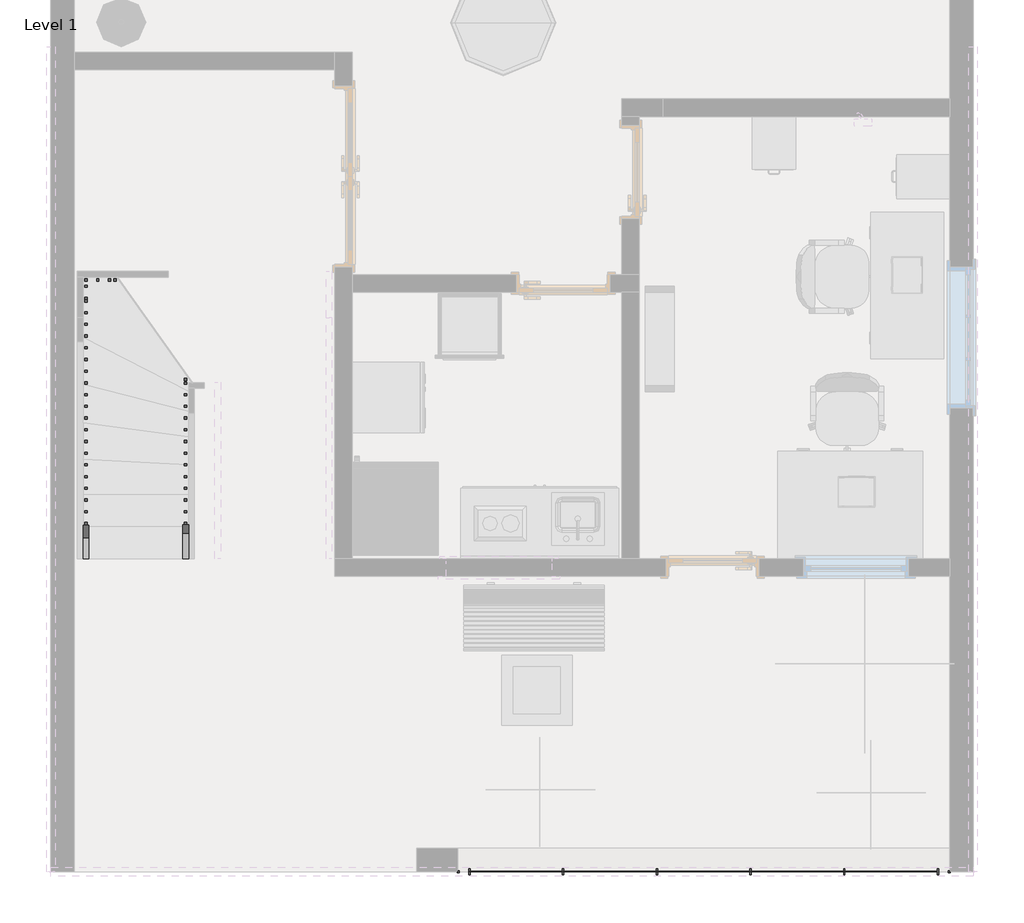
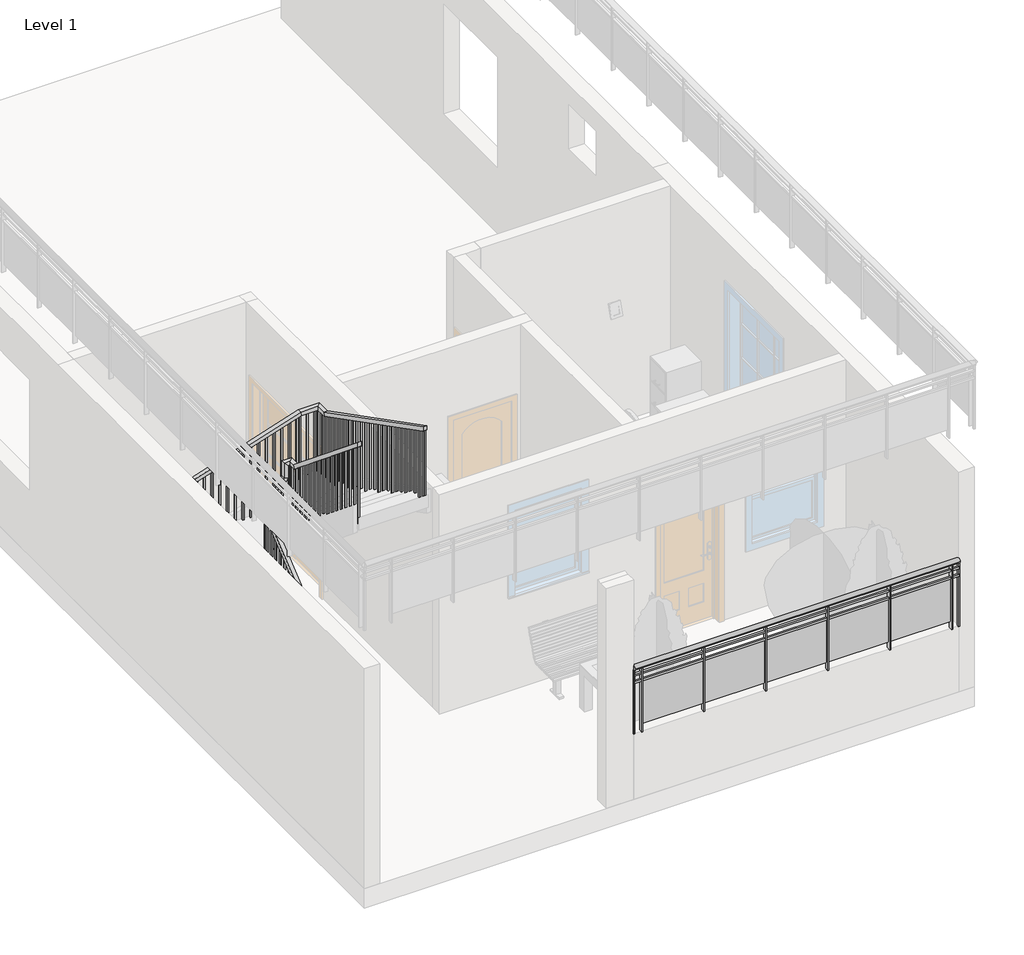
# One storey, part 2 of 4: 3 railings.
"""IFC4 building model written with IfcOpenShell, lengths in millimetres."""

from ifc_helpers import new_model, si_unit, point, frame, origin, place, context, project, spatial, polyline, ellipse_curve, trimmed, outline, extrude, faceted_brep, element, save
from ifc_brep_helpers import plane_surface, extruded_surface, advanced_brep

model = new_model("IFC4")

# Units and contexts
model_context = context("Model", 3, world=origin())
ifc_project = project(units=[si_unit("LENGTHUNIT", "METRE", prefix="MILLI")], contexts=[model_context])

# Site, building, storey
site = spatial("IfcSite", under=ifc_project)
building = spatial("IfcBuilding", under=site)
storey = spatial("IfcBuildingStorey", under=building, Name="Level 1", Elevation=0.0)

# Railings
placement = place(None, origin())
element("IfcRailing", 1, ObjectType="Glass Panel - Bottom Fill", at=placement, inside=storey, context=model_context, shape_type="SolidModel", body=[
    advanced_brep(
    [(-10033.9568901, -1887.378876, 1828.8), (-10033.9568901, -1963.578876, 1828.8), (-5766.7568901, -1887.378876, 1828.8), (-5766.7568901, -1963.578876, 1828.8)],
    [
        (0, 1, ellipse_curve(frame((-10033.9568901, -1925.478876, 1828.8), z_axis=(-1.0, 0.0, 0.0), x_axis=(0.0, -1.0, 0.0)), 38.1, 28.575)),
        (1, 0, ellipse_curve(frame((-10033.9568901, -1925.478876, 1828.8), z_axis=(-1.0, 0.0, 0.0), x_axis=(0.0, -1.0, 0.0)), 38.1, 28.575)),
        (2, 3, ellipse_curve(frame((-5766.7568901, -1925.478876, 1828.8), z_axis=(1.0, 0.0, 0.0), x_axis=(0.0, -1.0, 0.0)), 38.1, 28.575)),
        (3, 2, ellipse_curve(frame((-5766.7568901, -1925.478876, 1828.8), z_axis=(1.0, 0.0, 0.0), x_axis=(0.0, -1.0, 0.0)), 38.1, 28.575)),
        (0, 2),
        (3, 1),
    ],
    [
        plane_surface(frame((-10033.9568901, -1925.478876, 1828.8), z_axis=(-1.0, 0.0, 0.0), x_axis=(0.0, 1.0, 0.0))),
        plane_surface(frame((-5766.7568901, -1925.478876, 1828.8), z_axis=(1.0, 0.0, 0.0), x_axis=(0.0, 1.0, 0.0))),
        extruded_surface(trimmed(ellipse_curve(frame((-5766.7568901, -1925.478876, 1828.8), z_axis=(-1.0, 0.0, 0.0), x_axis=(0.0, -1.0, 0.0)), 38.1, 28.575), [point((-5766.7568901, -1887.378876, 1828.8))], [point((-5766.7568901, -1963.578876, 1828.8))], True, "CARTESIAN"), (-4267.2, 0.0, 0.0), 4267.2),
        extruded_surface(trimmed(ellipse_curve(frame((-5766.7568901, -1925.478876, 1828.8), z_axis=(-1.0, 0.0, 0.0), x_axis=(0.0, -1.0, 0.0)), 38.1, 28.575), [point((-5766.7568901, -1963.578876, 1828.8))], [point((-5766.7568901, -1887.378876, 1828.8))], True, "CARTESIAN"), (-4267.2, 0.0, 0.0), 4267.2),
    ],
    [
        (0, [[1, 2]]),
        (1, [[3, 4]]),
        (2, [[-1, 5, -4, 6]]),
        (3, [[-2, -6, -3, -5]]),
    ],
),
    extrude(outline(polyline([(-10033.9568901, -1938.178876), (-10033.9568901, -1912.778876), (-5766.7568901, -1912.778876), (-5766.7568901, -1938.178876), (-10033.9568901, -1938.178876)])), frame((0.0, 0.0, 1714.5), z_axis=(0.0, 0.0, 1.0), x_axis=(1.0, 0.0, 0.0)), (0.0, 0.0, 1.0), 25.4),
    extrude(outline(polyline([(-10033.9568901, -1938.178876), (-10033.9568901, -1912.778876), (-5766.7568901, -1912.778876), (-5766.7568901, -1938.178876), (-10033.9568901, -1938.178876)])), frame((0.0, 0.0, 1612.9), z_axis=(0.0, 0.0, 1.0), x_axis=(1.0, 0.0, 0.0)), (0.0, 0.0, 1.0), 25.4),
    extrude(outline(polyline([(-5874.7068901, -1950.878876), (-5874.7068901, -1900.078876), (-5862.0068901, -1900.078876), (-5862.0068901, -1950.878876), (-5874.7068901, -1950.878876)])), frame((0.0, 0.0, 914.4), z_axis=(0.0, 0.0, 1.0), x_axis=(1.0, 0.0, 0.0)), (0.0, 0.0, 1.0), 885.6788223),
    extrude(outline(polyline([(-6681.1568901, -1918.943719), (-5868.3568901, -1918.943719), (-5868.3568901, -1925.293719), (-6681.1568901, -1925.293719), (-6681.1568901, -1918.943719)])), frame((0.0, 0.0, 1016.0), z_axis=(0.0, 0.0, 1.0), x_axis=(1.0, 0.0, 0.0)), (0.0, 0.0, 1.0), 596.9),
    extrude(outline(polyline([(-6687.5068901, -1950.878876), (-6687.5068901, -1900.078876), (-6674.8068901, -1900.078876), (-6674.8068901, -1950.878876), (-6687.5068901, -1950.878876)])), frame((0.0, 0.0, 914.4), z_axis=(0.0, 0.0, 1.0), x_axis=(1.0, 0.0, 0.0)), (0.0, 0.0, 1.0), 885.6788223),
    extrude(outline(polyline([(-7493.9568901, -1918.943719), (-6681.1568901, -1918.943719), (-6681.1568901, -1925.293719), (-7493.9568901, -1925.293719), (-7493.9568901, -1918.943719)])), frame((0.0, 0.0, 1016.0), z_axis=(0.0, 0.0, 1.0), x_axis=(1.0, 0.0, 0.0)), (0.0, 0.0, 1.0), 596.9),
    extrude(outline(polyline([(-7500.3068901, -1950.878876), (-7500.3068901, -1900.078876), (-7487.6068901, -1900.078876), (-7487.6068901, -1950.878876), (-7500.3068901, -1950.878876)])), frame((0.0, 0.0, 914.4), z_axis=(0.0, 0.0, 1.0), x_axis=(1.0, 0.0, 0.0)), (0.0, 0.0, 1.0), 885.6788223),
    extrude(outline(polyline([(-8306.7568901, -1918.943719), (-7493.9568901, -1918.943719), (-7493.9568901, -1925.293719), (-8306.7568901, -1925.293719), (-8306.7568901, -1918.943719)])), frame((0.0, 0.0, 1016.0), z_axis=(0.0, 0.0, 1.0), x_axis=(1.0, 0.0, 0.0)), (0.0, 0.0, 1.0), 596.9),
    extrude(outline(polyline([(-8313.1068901, -1950.878876), (-8313.1068901, -1900.078876), (-8300.4068901, -1900.078876), (-8300.4068901, -1950.878876), (-8313.1068901, -1950.878876)])), frame((0.0, 0.0, 914.4), z_axis=(0.0, 0.0, 1.0), x_axis=(1.0, 0.0, 0.0)), (0.0, 0.0, 1.0), 885.6788223),
    extrude(outline(polyline([(-9119.5568901, -1918.943719), (-8306.7568901, -1918.943719), (-8306.7568901, -1925.293719), (-9119.5568901, -1925.293719), (-9119.5568901, -1918.943719)])), frame((0.0, 0.0, 1016.0), z_axis=(0.0, 0.0, 1.0), x_axis=(1.0, 0.0, 0.0)), (0.0, 0.0, 1.0), 596.9),
    extrude(outline(polyline([(-9125.9068901, -1950.878876), (-9125.9068901, -1900.078876), (-9113.2068901, -1900.078876), (-9113.2068901, -1950.878876), (-9125.9068901, -1950.878876)])), frame((0.0, 0.0, 914.4), z_axis=(0.0, 0.0, 1.0), x_axis=(1.0, 0.0, 0.0)), (0.0, 0.0, 1.0), 885.6788223),
    extrude(outline(polyline([(-9932.3568901, -1918.943719), (-9119.5568901, -1918.943719), (-9119.5568901, -1925.293719), (-9932.3568901, -1925.293719), (-9932.3568901, -1918.943719)])), frame((0.0, 0.0, 1016.0), z_axis=(0.0, 0.0, 1.0), x_axis=(1.0, 0.0, 0.0)), (0.0, 0.0, 1.0), 596.9),
    extrude(outline(polyline([(-9938.7068901, -1950.878876), (-9938.7068901, -1900.078876), (-9926.0068901, -1900.078876), (-9926.0068901, -1950.878876), (-9938.7068901, -1950.878876)])), frame((0.0, 0.0, 914.4), z_axis=(0.0, 0.0, 1.0), x_axis=(1.0, 0.0, 0.0)), (0.0, 0.0, 1.0), 885.6788223),
    extrude(outline(polyline([(-5779.4568901, -1935.003876), (-5779.4568901, -1915.953876), (-5760.4068901, -1915.953876), (-5760.4068901, -1935.003876), (-5779.4568901, -1935.003876)])), frame((0.0, 0.0, 914.4), z_axis=(0.0, 0.0, 1.0), x_axis=(1.0, 0.0, 0.0)), (0.0, 0.0, 1.0), 885.6788223),
    extrude(outline(polyline([(-10040.3068901, -1935.003876), (-10040.3068901, -1915.953876), (-10021.2568901, -1915.953876), (-10021.2568901, -1935.003876), (-10040.3068901, -1935.003876)])), frame((0.0, 0.0, 914.4), z_axis=(0.0, 0.0, 1.0), x_axis=(1.0, 0.0, 0.0)), (0.0, 0.0, 1.0), 885.6788223),
])
element("IfcRailing", 2, ObjectType="Handrail - Rectangular", at=placement, inside=storey, context=model_context, shape_type="SolidModel", body=[
    faceted_brep([(-12421.5568901, 792.321124, 1025.2529681), (-12421.5568901, 792.321124, 959.7067088), (-12370.7568901, 792.321124, 959.7067088), (-12370.7568901, 792.321124, 1025.2529681), (-12421.5568901, 2243.8528159, 2208.7848338), (-12421.5568901, 2294.6528159, 2184.659247), (-12370.7568901, 2294.6528159, 2184.659247), (-12370.7568901, 2243.8528159, 2208.7848338), (-12421.5568901, 2243.8528159, 2414.6281882), (-12421.5568901, 2294.6528159, 2363.8281882), (-12370.7568901, 2294.6528159, 2363.8281882), (-12370.7568901, 2243.8528159, 2414.6281882), (-12421.5568901, 2370.8528159, 2414.6281882), (-12421.5568901, 2370.8528159, 2363.8281882), (-12370.7568901, 2320.0528159, 2363.8281882), (-12370.7568901, 2320.0528159, 2414.6281882), (-12294.5568901, 2370.8528159, 2414.6281882), (-12265.4355563, 2370.8528159, 2363.8281882), (-12265.4355563, 2320.0528159, 2363.8281882), (-12294.5568901, 2320.0528159, 2414.6281882), (-12167.5568901, 2370.8528159, 2631.5051451), (-12116.7568901, 2370.8528159, 2617.7256424), (-12116.7568901, 2320.0528159, 2617.7256424), (-12167.5568901, 2320.0528159, 2631.5051451), (-12167.5568901, 2370.8528159, 2837.3484995), (-12116.7568901, 2370.8528159, 2786.5484995), (-12116.7568901, 2320.0528159, 2786.5484995), (-12167.5568901, 2320.0528159, 2837.3484995), (-12040.5568901, 2370.8528159, 2837.3484995), (-12040.5568901, 2370.8528159, 2786.5484995), (-12091.3568901, 2320.0528159, 2786.5484995), (-12091.3568901, 2320.0528159, 2837.3484995), (-12040.5568901, 2243.8528159, 2837.3484995), (-12040.5568901, 2225.7674028, 2786.5484995), (-12091.3568901, 2225.7674028, 2786.5484995), (-12091.3568901, 2243.8528159, 2837.3484995), (-12040.5568901, 792.321124, 4020.8803652), (-12091.3568901, 792.321124, 4020.8803652), (-12091.3568901, 792.321124, 3955.3341059), (-12040.5568901, 792.321124, 3955.3341059)], [[[0, 1, 2, 3]], [[1, 0, 4, 5]], [[2, 1, 5, 6]], [[3, 2, 6, 7]], [[0, 3, 7, 4]], [[5, 4, 8, 9]], [[6, 5, 9, 10]], [[7, 6, 10, 11]], [[4, 7, 11, 8]], [[9, 8, 12, 13]], [[10, 9, 13, 14]], [[11, 10, 14, 15]], [[8, 11, 15, 12]], [[13, 12, 16, 17]], [[14, 13, 17, 18]], [[15, 14, 18, 19]], [[12, 15, 19, 16]], [[17, 16, 20, 21]], [[18, 17, 21, 22]], [[19, 18, 22, 23]], [[16, 19, 23, 20]], [[21, 20, 24, 25]], [[22, 21, 25, 26]], [[23, 22, 26, 27]], [[20, 23, 27, 24]], [[25, 24, 28, 29]], [[26, 25, 29, 30]], [[27, 26, 30, 31]], [[24, 27, 31, 28]], [[29, 28, 32, 33]], [[30, 29, 33, 34]], [[31, 30, 34, 35]], [[28, 31, 35, 32]], [[36, 37, 38, 39]], [[33, 32, 36, 39]], [[34, 33, 39, 38]], [[35, 34, 38, 37]], [[32, 35, 37, 36]]]),
    extrude(outline(polyline([(882.5604595, 3881.7558784), (901.6104595, 3866.2231262), (901.6104595, 2878.6666667), (882.5604595, 2878.6666667), (882.5604595, 3881.7558784)])), frame((-12075.4818901, 0.0, 0.0), z_axis=(1.0, 0.0, 0.0), x_axis=(0.0, 1.0, 0.0)), (0.0, 0.0, 1.0), 19.05),
    extrude(outline(polyline([(984.1604595, 3798.9145334), (1003.2104595, 3783.3817813), (1003.2104595, 2878.6666667), (984.1604595, 2878.6666667), (984.1604595, 3798.9145334)])), frame((-12075.4818901, 0.0, 0.0), z_axis=(1.0, 0.0, 0.0), x_axis=(0.0, 1.0, 0.0)), (0.0, 0.0, 1.0), 19.05),
    extrude(outline(polyline([(1085.7604595, 3716.0731885), (1104.8104595, 3700.5404364), (1104.8104595, 2709.3333333), (1085.7604595, 2709.3333333), (1085.7604595, 3716.0731885)])), frame((-12075.4818901, 0.0, 0.0), z_axis=(1.0, 0.0, 0.0), x_axis=(0.0, 1.0, 0.0)), (0.0, 0.0, 1.0), 19.05),
    extrude(outline(polyline([(1187.3604595, 3633.2318436), (1206.4104595, 3617.6990914), (1206.4104595, 2709.3333333), (1187.3604595, 2709.3333333), (1187.3604595, 3633.2318436)])), frame((-12075.4818901, 0.0, 0.0), z_axis=(1.0, 0.0, 0.0), x_axis=(0.0, 1.0, 0.0)), (0.0, 0.0, 1.0), 19.05),
    extrude(outline(polyline([(1288.9604595, 3550.3904987), (1308.0104595, 3534.8577465), (1308.0104595, 2709.3333333), (1288.9604595, 2709.3333333), (1288.9604595, 3550.3904987)])), frame((-12075.4818901, 0.0, 0.0), z_axis=(1.0, 0.0, 0.0), x_axis=(0.0, 1.0, 0.0)), (0.0, 0.0, 1.0), 19.05),
    extrude(outline(polyline([(1390.5604595, 3467.5491538), (1409.6104595, 3452.0164016), (1409.6104595, 2540.0), (1390.5604595, 2540.0), (1390.5604595, 3467.5491538)])), frame((-12075.4818901, 0.0, 0.0), z_axis=(1.0, 0.0, 0.0), x_axis=(0.0, 1.0, 0.0)), (0.0, 0.0, 1.0), 19.05),
    extrude(outline(polyline([(1492.1604595, 3384.7078088), (1511.2104595, 3369.1750567), (1511.2104595, 2540.0), (1492.1604595, 2540.0), (1492.1604595, 3384.7078088)])), frame((-12075.4818901, 0.0, 0.0), z_axis=(1.0, 0.0, 0.0), x_axis=(0.0, 1.0, 0.0)), (0.0, 0.0, 1.0), 19.05),
    extrude(outline(polyline([(1593.7604595, 3301.8664639), (1612.8104595, 3286.3337117), (1612.8104595, 2540.0), (1593.7604595, 2540.0), (1593.7604595, 3301.8664639)])), frame((-12075.4818901, 0.0, 0.0), z_axis=(1.0, 0.0, 0.0), x_axis=(0.0, 1.0, 0.0)), (0.0, 0.0, 1.0), 19.05),
    extrude(outline(polyline([(1695.3604595, 3219.025119), (1714.4104595, 3203.4923668), (1714.4104595, 2370.6666667), (1695.3604595, 2370.6666667), (1695.3604595, 3219.025119)])), frame((-12075.4818901, 0.0, 0.0), z_axis=(1.0, 0.0, 0.0), x_axis=(0.0, 1.0, 0.0)), (0.0, 0.0, 1.0), 19.05),
    extrude(outline(polyline([(1796.9604595, 3136.1837741), (1816.0104595, 3120.6510219), (1816.0104595, 2370.6666667), (1796.9604595, 2370.6666667), (1796.9604595, 3136.1837741)])), frame((-12075.4818901, 0.0, 0.0), z_axis=(1.0, 0.0, 0.0), x_axis=(0.0, 1.0, 0.0)), (0.0, 0.0, 1.0), 19.05),
    extrude(outline(polyline([(1898.5604595, 3053.3424291), (1917.6104595, 3037.809677), (1917.6104595, 2201.3333333), (1898.5604595, 2201.3333333), (1898.5604595, 3053.3424291)])), frame((-12075.4818901, 0.0, 0.0), z_axis=(1.0, 0.0, 0.0), x_axis=(0.0, 1.0, 0.0)), (0.0, 0.0, 1.0), 19.05),
    extrude(outline(polyline([(2000.1604595, 2970.5010842), (2019.2104595, 2954.9683321), (2019.2104595, 2201.3333333), (2000.1604595, 2201.3333333), (2000.1604595, 2970.5010842)])), frame((-12075.4818901, 0.0, 0.0), z_axis=(1.0, 0.0, 0.0), x_axis=(0.0, 1.0, 0.0)), (0.0, 0.0, 1.0), 19.05),
    extrude(outline(polyline([(2101.7604595, 2887.6597393), (2120.8104595, 2872.1269871), (2120.8104595, 2032.0), (2101.7604595, 2032.0), (2101.7604595, 2887.6597393)])), frame((-12075.4818901, 0.0, 0.0), z_axis=(1.0, 0.0, 0.0), x_axis=(0.0, 1.0, 0.0)), (0.0, 0.0, 1.0), 19.05),
    extrude(outline(polyline([(2203.3604595, 2804.8183944), (2222.4104595, 2789.2856422), (2222.4104595, 2032.0), (2203.3604595, 2032.0), (2203.3604595, 2804.8183944)])), frame((-12075.4818901, 0.0, 0.0), z_axis=(1.0, 0.0, 0.0), x_axis=(0.0, 1.0, 0.0)), (0.0, 0.0, 1.0), 19.05),
    extrude(outline(polyline([(2529.115018, -12168.6459863), (2496.5834745, -12187.6959863), (1524.0, -12187.6959863), (1524.0, -12168.6459863), (2529.115018, -12168.6459863)])), frame((0.0, 2335.9278159, 0.0), z_axis=(0.0, 1.0, 0.0), x_axis=(0.0, 0.0, 1.0)), (0.0, 0.0, 1.0), 19.05),
    extrude(outline(polyline([(2355.6134525, -12270.2459863), (2323.0819089, -12289.2959863), (1524.0, -12289.2959863), (1524.0, -12270.2459863), (2355.6134525, -12270.2459863)])), frame((0.0, 2335.9278159, 0.0), z_axis=(0.0, 1.0, 0.0), x_axis=(0.0, 0.0, 1.0)), (0.0, 0.0, 1.0), 19.05),
    extrude(outline(polyline([(2205.196124, 2111.7191617), (2224.246124, 2127.2519138), (2224.246124, 1016.0), (2205.196124, 1016.0), (2205.196124, 2111.7191617)])), frame((-12405.6818901, 0.0, 0.0), z_axis=(1.0, 0.0, 0.0), x_axis=(0.0, 1.0, 0.0)), (0.0, 0.0, 1.0), 19.05),
    extrude(outline(polyline([(2103.596124, 2028.8778167), (2122.646124, 2044.4105689), (2122.646124, 1016.0), (2103.596124, 1016.0), (2103.596124, 2028.8778167)])), frame((-12405.6818901, 0.0, 0.0), z_axis=(1.0, 0.0, 0.0), x_axis=(0.0, 1.0, 0.0)), (0.0, 0.0, 1.0), 19.05),
    extrude(outline(polyline([(2001.996124, 1946.0364718), (2021.046124, 1961.569224), (2021.046124, 846.6666667), (2001.996124, 846.6666667), (2001.996124, 1946.0364718)])), frame((-12405.6818901, 0.0, 0.0), z_axis=(1.0, 0.0, 0.0), x_axis=(0.0, 1.0, 0.0)), (0.0, 0.0, 1.0), 19.05),
    extrude(outline(polyline([(1900.396124, 1863.1951269), (1919.446124, 1878.7278791), (1919.446124, 846.6666667), (1900.396124, 846.6666667), (1900.396124, 1863.1951269)])), frame((-12405.6818901, 0.0, 0.0), z_axis=(1.0, 0.0, 0.0), x_axis=(0.0, 1.0, 0.0)), (0.0, 0.0, 1.0), 19.05),
    extrude(outline(polyline([(1798.796124, 1780.353782), (1817.846124, 1795.8865341), (1817.846124, 677.3333333), (1798.796124, 677.3333333), (1798.796124, 1780.353782)])), frame((-12405.6818901, 0.0, 0.0), z_axis=(1.0, 0.0, 0.0), x_axis=(0.0, 1.0, 0.0)), (0.0, 0.0, 1.0), 19.05),
    extrude(outline(polyline([(1697.196124, 1697.5124371), (1716.246124, 1713.0451892), (1716.246124, 677.3333333), (1697.196124, 677.3333333), (1697.196124, 1697.5124371)])), frame((-12405.6818901, 0.0, 0.0), z_axis=(1.0, 0.0, 0.0), x_axis=(0.0, 1.0, 0.0)), (0.0, 0.0, 1.0), 19.05),
    extrude(outline(polyline([(1595.596124, 1614.6710921), (1614.646124, 1630.2038443), (1614.646124, 508.0), (1595.596124, 508.0), (1595.596124, 1614.6710921)])), frame((-12405.6818901, 0.0, 0.0), z_axis=(1.0, 0.0, 0.0), x_axis=(0.0, 1.0, 0.0)), (0.0, 0.0, 1.0), 19.05),
    extrude(outline(polyline([(1493.996124, 1531.8297472), (1513.046124, 1547.3624994), (1513.046124, 508.0), (1493.996124, 508.0), (1493.996124, 1531.8297472)])), frame((-12405.6818901, 0.0, 0.0), z_axis=(1.0, 0.0, 0.0), x_axis=(0.0, 1.0, 0.0)), (0.0, 0.0, 1.0), 19.05),
    extrude(outline(polyline([(1392.396124, 1448.9884023), (1411.446124, 1464.5211545), (1411.446124, 508.0), (1392.396124, 508.0), (1392.396124, 1448.9884023)])), frame((-12405.6818901, 0.0, 0.0), z_axis=(1.0, 0.0, 0.0), x_axis=(0.0, 1.0, 0.0)), (0.0, 0.0, 1.0), 19.05),
    extrude(outline(polyline([(1290.796124, 1366.1470574), (1309.846124, 1381.6798095), (1309.846124, 338.6666667), (1290.796124, 338.6666667), (1290.796124, 1366.1470574)])), frame((-12405.6818901, 0.0, 0.0), z_axis=(1.0, 0.0, 0.0), x_axis=(0.0, 1.0, 0.0)), (0.0, 0.0, 1.0), 19.05),
    extrude(outline(polyline([(1189.196124, 1283.3057124), (1208.246124, 1298.8384646), (1208.246124, 338.6666667), (1189.196124, 338.6666667), (1189.196124, 1283.3057124)])), frame((-12405.6818901, 0.0, 0.0), z_axis=(1.0, 0.0, 0.0), x_axis=(0.0, 1.0, 0.0)), (0.0, 0.0, 1.0), 19.05),
    extrude(outline(polyline([(1087.596124, 1200.4643675), (1106.646124, 1215.9971197), (1106.646124, 338.6666667), (1087.596124, 338.6666667), (1087.596124, 1200.4643675)])), frame((-12405.6818901, 0.0, 0.0), z_axis=(1.0, 0.0, 0.0), x_axis=(0.0, 1.0, 0.0)), (0.0, 0.0, 1.0), 19.05),
    extrude(outline(polyline([(985.996124, 1117.6230226), (1005.046124, 1133.1557748), (1005.046124, 169.3333333), (985.996124, 169.3333333), (985.996124, 1117.6230226)])), frame((-12405.6818901, 0.0, 0.0), z_axis=(1.0, 0.0, 0.0), x_axis=(0.0, 1.0, 0.0)), (0.0, 0.0, 1.0), 19.05),
    extrude(outline(polyline([(884.396124, 1034.7816777), (903.446124, 1050.3144298), (903.446124, 169.3333333), (884.396124, 169.3333333), (884.396124, 1034.7816777)])), frame((-12405.6818901, 0.0, 0.0), z_axis=(1.0, 0.0, 0.0), x_axis=(0.0, 1.0, 0.0)), (0.0, 0.0, 1.0), 19.05),
    extrude(outline(polyline([(-12075.4818901, 2324.0104595), (-12056.4318901, 2324.0104595), (-12056.4318901, 2304.9604595), (-12075.4818901, 2304.9604595), (-12075.4818901, 2324.0104595)])), frame((0.0, 0.0, 1862.6666667), z_axis=(0.0, 0.0, 1.0), x_axis=(1.0, 0.0, 0.0)), (0.0, 0.0, 1.0), 923.8818329),
    extrude(outline(polyline([(-12075.4818901, 2335.9278159), (-12075.4818901, 2354.9778159), (-12056.4318901, 2354.9778159), (-12056.4318901, 2335.9278159), (-12075.4818901, 2335.9278159)])), frame((0.0, 0.0, 1862.6666667), z_axis=(0.0, 0.0, 1.0), x_axis=(1.0, 0.0, 0.0)), (0.0, 0.0, 1.0), 923.8818329),
    extrude(outline(polyline([(-12090.2677938, 2335.9278159), (-12090.2677938, 2354.9778159), (-12071.2177938, 2354.9778159), (-12071.2177938, 2335.9278159), (-12090.2677938, 2335.9278159)])), frame((0.0, 0.0, 1693.3333333), z_axis=(0.0, 0.0, 1.0), x_axis=(1.0, 0.0, 0.0)), (0.0, 0.0, 1.0), 1093.2151662),
    extrude(outline(polyline([(-12390.8959863, 2335.9278159), (-12390.8959863, 2354.9778159), (-12371.8459863, 2354.9778159), (-12371.8459863, 2335.9278159), (-12390.8959863, 2335.9278159)])), frame((0.0, 0.0, 1354.6666667), z_axis=(0.0, 0.0, 1.0), x_axis=(1.0, 0.0, 0.0)), (0.0, 0.0, 1.0), 1009.1615215),
    extrude(outline(polyline([(-12386.6318901, 2335.9278159), (-12405.6818901, 2335.9278159), (-12405.6818901, 2354.9778159), (-12386.6318901, 2354.9778159), (-12386.6318901, 2335.9278159)])), frame((0.0, 0.0, 1185.3333333), z_axis=(0.0, 0.0, 1.0), x_axis=(1.0, 0.0, 0.0)), (0.0, 0.0, 1.0), 1178.4948549),
    extrude(outline(polyline([(-12386.6318901, 2304.9604595), (-12405.6818901, 2304.9604595), (-12405.6818901, 2324.0104595), (-12386.6318901, 2324.0104595), (-12386.6318901, 2304.9604595)])), frame((0.0, 0.0, 1185.3333333), z_axis=(0.0, 0.0, 1.0), x_axis=(1.0, 0.0, 0.0)), (0.0, 0.0, 1.0), 1178.4948549),
    extrude(outline(polyline([(792.321124, 3955.3341059), (811.371124, 3939.8013537), (811.371124, 2878.6666667), (792.321124, 2878.6666667), (792.321124, 3955.3341059)])), frame((-12075.4818901, 0.0, 0.0), z_axis=(1.0, 0.0, 0.0), x_axis=(0.0, 1.0, 0.0)), (0.0, 0.0, 1.0), 19.05),
    extrude(outline(polyline([(792.321124, 959.7067088), (811.371124, 975.239461), (811.371124, 169.3333333), (792.321124, 169.3333333), (792.321124, 959.7067088)])), frame((-12405.6818901, 0.0, 0.0), z_axis=(1.0, 0.0, 0.0), x_axis=(0.0, 1.0, 0.0)), (0.0, 0.0, 1.0), 19.05),
])
element("IfcRailing", 3, ObjectType="Handrail - Rectangular", at=placement, inside=storey, context=model_context, shape_type="SolidModel", body=[
    faceted_brep([(-13285.1568901, 792.321124, 1109.0771751), (-13285.1568901, 792.321124, 1051.9280057), (-13234.3568901, 792.321124, 1051.9280057), (-13234.3568901, 792.321124, 1109.0771751), (-13285.1568901, 3052.3029805, 2273.7644996), (-13285.1568901, 3064.6230318, 2222.9644996), (-13234.3568901, 3064.6230318, 2222.9644996), (-13234.3568901, 3052.3029805, 2273.7644996), (-13285.1568901, 3234.4528159, 2273.7644996), (-13285.1568901, 3234.4528159, 2222.9644996), (-13234.3568901, 3183.6528159, 2222.9644996), (-13234.3568901, 3183.6528159, 2273.7644996), (-13008.0029375, 3234.4528159, 2273.7644996), (-13000.0523613, 3234.4528159, 2222.9644996), (-13000.0523613, 3183.6528159, 2222.9644996), (-13008.0029375, 3183.6528159, 2273.7644996), (-11454.1108427, 3234.4528159, 2772.3688337), (-11446.1602666, 3234.4528159, 2721.5688337), (-11446.1602666, 3183.6528159, 2721.5688337), (-11454.1108427, 3183.6528159, 2772.3688337), (-11176.9568901, 3234.4528159, 2772.3688337), (-11176.9568901, 3234.4528159, 2721.5688337), (-11227.7568901, 3183.6528159, 2721.5688337), (-11227.7568901, 3183.6528159, 2772.3688337), (-11176.9568901, 3052.3029805, 2772.3688337), (-11176.9568901, 3039.9829292, 2721.5688337), (-11227.7568901, 3039.9829292, 2721.5688337), (-11227.7568901, 3052.3029805, 2772.3688337), (-11176.9568901, 792.321124, 3937.0561582), (-11227.7568901, 792.321124, 3937.0561582), (-11227.7568901, 792.321124, 3879.9069889), (-11176.9568901, 792.321124, 3879.9069889)], [[[0, 1, 2, 3]], [[1, 0, 4, 5]], [[2, 1, 5, 6]], [[3, 2, 6, 7]], [[0, 3, 7, 4]], [[5, 4, 8, 9]], [[6, 5, 9, 10]], [[7, 6, 10, 11]], [[4, 7, 11, 8]], [[9, 8, 12, 13]], [[10, 9, 13, 14]], [[11, 10, 14, 15]], [[8, 11, 15, 12]], [[13, 12, 16, 17]], [[14, 13, 17, 18]], [[15, 14, 18, 19]], [[12, 15, 19, 16]], [[17, 16, 20, 21]], [[18, 17, 21, 22]], [[19, 18, 22, 23]], [[16, 19, 23, 20]], [[21, 20, 24, 25]], [[22, 21, 25, 26]], [[23, 22, 26, 27]], [[20, 23, 27, 24]], [[28, 29, 30, 31]], [[25, 24, 28, 31]], [[26, 25, 31, 30]], [[27, 26, 30, 29]], [[24, 27, 29, 28]]]),
    extrude(outline(polyline([(826.6279805, 3862.2268642), (826.6279805, 2878.6666667), (807.5779805, 2878.6666667), (807.5779805, 3872.0443296), (826.6279805, 3862.2268642)])), frame((-11211.8818901, 0.0, 0.0), z_axis=(1.0, 0.0, 0.0), x_axis=(0.0, 1.0, 0.0)), (0.0, 0.0, 1.0), 19.05),
    extrude(outline(polyline([(928.2279805, 3809.8670491), (928.2279805, 2878.6666667), (909.1779805, 2878.6666667), (909.1779805, 3819.6845145), (928.2279805, 3809.8670491)])), frame((-11211.8818901, 0.0, 0.0), z_axis=(1.0, 0.0, 0.0), x_axis=(0.0, 1.0, 0.0)), (0.0, 0.0, 1.0), 19.05),
    extrude(outline(polyline([(1029.8279805, 3757.507234), (1029.8279805, 2878.6666667), (1010.7779805, 2878.6666667), (1010.7779805, 3767.3246993), (1029.8279805, 3757.507234)])), frame((-11211.8818901, 0.0, 0.0), z_axis=(1.0, 0.0, 0.0), x_axis=(0.0, 1.0, 0.0)), (0.0, 0.0, 1.0), 19.05),
    extrude(outline(polyline([(1131.4279805, 3705.1474189), (1131.4279805, 2709.3333333), (1112.3779805, 2709.3333333), (1112.3779805, 3714.9648842), (1131.4279805, 3705.1474189)])), frame((-11211.8818901, 0.0, 0.0), z_axis=(1.0, 0.0, 0.0), x_axis=(0.0, 1.0, 0.0)), (0.0, 0.0, 1.0), 19.05),
    extrude(outline(polyline([(1233.0279805, 3652.7876038), (1233.0279805, 2709.3333333), (1213.9779805, 2709.3333333), (1213.9779805, 3662.6050691), (1233.0279805, 3652.7876038)])), frame((-11211.8818901, 0.0, 0.0), z_axis=(1.0, 0.0, 0.0), x_axis=(0.0, 1.0, 0.0)), (0.0, 0.0, 1.0), 19.05),
    extrude(outline(polyline([(1334.6279805, 3600.4277887), (1334.6279805, 2709.3333333), (1315.5779805, 2709.3333333), (1315.5779805, 3610.245254), (1334.6279805, 3600.4277887)])), frame((-11211.8818901, 0.0, 0.0), z_axis=(1.0, 0.0, 0.0), x_axis=(0.0, 1.0, 0.0)), (0.0, 0.0, 1.0), 19.05),
    extrude(outline(polyline([(1436.2279805, 3548.0679735), (1436.2279805, 2540.0), (1417.1779805, 2540.0), (1417.1779805, 3557.8854389), (1436.2279805, 3548.0679735)])), frame((-11211.8818901, 0.0, 0.0), z_axis=(1.0, 0.0, 0.0), x_axis=(0.0, 1.0, 0.0)), (0.0, 0.0, 1.0), 19.05),
    extrude(outline(polyline([(1537.8279805, 3495.7081584), (1537.8279805, 2540.0), (1518.7779805, 2540.0), (1518.7779805, 3505.5256238), (1537.8279805, 3495.7081584)])), frame((-11211.8818901, 0.0, 0.0), z_axis=(1.0, 0.0, 0.0), x_axis=(0.0, 1.0, 0.0)), (0.0, 0.0, 1.0), 19.05),
    extrude(outline(polyline([(1639.4279805, 3443.3483433), (1639.4279805, 2540.0), (1620.3779805, 2540.0), (1620.3779805, 3453.1658086), (1639.4279805, 3443.3483433)])), frame((-11211.8818901, 0.0, 0.0), z_axis=(1.0, 0.0, 0.0), x_axis=(0.0, 1.0, 0.0)), (0.0, 0.0, 1.0), 19.05),
    extrude(outline(polyline([(1741.0279805, 3390.9885282), (1741.0279805, 2370.6666667), (1721.9779805, 2370.6666667), (1721.9779805, 3400.8059935), (1741.0279805, 3390.9885282)])), frame((-11211.8818901, 0.0, 0.0), z_axis=(1.0, 0.0, 0.0), x_axis=(0.0, 1.0, 0.0)), (0.0, 0.0, 1.0), 19.05),
    extrude(outline(polyline([(1842.6279805, 3338.6287131), (1842.6279805, 2370.6666667), (1823.5779805, 2370.6666667), (1823.5779805, 3348.4461784), (1842.6279805, 3338.6287131)])), frame((-11211.8818901, 0.0, 0.0), z_axis=(1.0, 0.0, 0.0), x_axis=(0.0, 1.0, 0.0)), (0.0, 0.0, 1.0), 19.05),
    extrude(outline(polyline([(1944.2279805, 3286.268898), (1944.2279805, 2370.6666667), (1925.1779805, 2370.6666667), (1925.1779805, 3296.0863633), (1944.2279805, 3286.268898)])), frame((-11211.8818901, 0.0, 0.0), z_axis=(1.0, 0.0, 0.0), x_axis=(0.0, 1.0, 0.0)), (0.0, 0.0, 1.0), 19.05),
    extrude(outline(polyline([(2045.8279805, 3233.9090828), (2045.8279805, 2201.3333333), (2026.7779805, 2201.3333333), (2026.7779805, 3243.7265482), (2045.8279805, 3233.9090828)])), frame((-11211.8818901, 0.0, 0.0), z_axis=(1.0, 0.0, 0.0), x_axis=(0.0, 1.0, 0.0)), (0.0, 0.0, 1.0), 19.05),
    extrude(outline(polyline([(2147.4279805, 3181.5492677), (2147.4279805, 2201.3333333), (2128.3779805, 2201.3333333), (2128.3779805, 3191.3667331), (2147.4279805, 3181.5492677)])), frame((-11211.8818901, 0.0, 0.0), z_axis=(1.0, 0.0, 0.0), x_axis=(0.0, 1.0, 0.0)), (0.0, 0.0, 1.0), 19.05),
    extrude(outline(polyline([(2249.0279805, 3129.1894526), (2249.0279805, 2201.3333333), (2229.9779805, 2201.3333333), (2229.9779805, 3139.0069179), (2249.0279805, 3129.1894526)])), frame((-11211.8818901, 0.0, 0.0), z_axis=(1.0, 0.0, 0.0), x_axis=(0.0, 1.0, 0.0)), (0.0, 0.0, 1.0), 19.05),
    extrude(outline(polyline([(2350.6279805, 3076.8296375), (2350.6279805, 2032.0), (2331.5779805, 2032.0), (2331.5779805, 3086.6471028), (2350.6279805, 3076.8296375)])), frame((-11211.8818901, 0.0, 0.0), z_axis=(1.0, 0.0, 0.0), x_axis=(0.0, 1.0, 0.0)), (0.0, 0.0, 1.0), 19.05),
    extrude(outline(polyline([(2452.2279805, 3024.4698224), (2452.2279805, 2032.0), (2433.1779805, 2032.0), (2433.1779805, 3034.2872877), (2452.2279805, 3024.4698224)])), frame((-11211.8818901, 0.0, 0.0), z_axis=(1.0, 0.0, 0.0), x_axis=(0.0, 1.0, 0.0)), (0.0, 0.0, 1.0), 19.05),
    extrude(outline(polyline([(2553.8279805, 2972.1100073), (2553.8279805, 2032.0), (2534.7779805, 2032.0), (2534.7779805, 2981.9274726), (2553.8279805, 2972.1100073)])), frame((-11211.8818901, 0.0, 0.0), z_axis=(1.0, 0.0, 0.0), x_axis=(0.0, 1.0, 0.0)), (0.0, 0.0, 1.0), 19.05),
    extrude(outline(polyline([(2655.4279805, 2919.7501921), (2655.4279805, 2032.0), (2636.3779805, 2032.0), (2636.3779805, 2929.5676575), (2655.4279805, 2919.7501921)])), frame((-11211.8818901, 0.0, 0.0), z_axis=(1.0, 0.0, 0.0), x_axis=(0.0, 1.0, 0.0)), (0.0, 0.0, 1.0), 19.05),
    extrude(outline(polyline([(2757.0279805, 2867.390377), (2757.0279805, 1862.6666667), (2737.9779805, 1862.6666667), (2737.9779805, 2877.2078424), (2757.0279805, 2867.390377)])), frame((-11211.8818901, 0.0, 0.0), z_axis=(1.0, 0.0, 0.0), x_axis=(0.0, 1.0, 0.0)), (0.0, 0.0, 1.0), 19.05),
    extrude(outline(polyline([(2858.6279805, 2815.0305619), (2858.6279805, 1862.6666667), (2839.5779805, 1862.6666667), (2839.5779805, 2824.8480272), (2858.6279805, 2815.0305619)])), frame((-11211.8818901, 0.0, 0.0), z_axis=(1.0, 0.0, 0.0), x_axis=(0.0, 1.0, 0.0)), (0.0, 0.0, 1.0), 19.05),
    extrude(outline(polyline([(2960.2279805, 2762.6707468), (2960.2279805, 1862.6666667), (2941.1779805, 1862.6666667), (2941.1779805, 2772.4882121), (2960.2279805, 2762.6707468)])), frame((-11211.8818901, 0.0, 0.0), z_axis=(1.0, 0.0, 0.0), x_axis=(0.0, 1.0, 0.0)), (0.0, 0.0, 1.0), 19.05),
    extrude(outline(polyline([(-11192.8318901, 3116.9778159), (-11192.8318901, 3097.9278159), (-11211.8818901, 3097.9278159), (-11211.8818901, 3116.9778159), (-11192.8318901, 3116.9778159)])), frame((0.0, 0.0, 1862.6666667), z_axis=(0.0, 0.0, 1.0), x_axis=(1.0, 0.0, 0.0)), (0.0, 0.0, 1.0), 858.902167),
    extrude(outline(polyline([(-11260.4358427, 3218.5778159), (-11241.3858427, 3218.5778159), (-11241.3858427, 3199.5278159), (-11260.4358427, 3199.5278159), (-11260.4358427, 3218.5778159)])), frame((0.0, 0.0, 1862.6666667), z_axis=(0.0, 0.0, 1.0), x_axis=(1.0, 0.0, 0.0)), (0.0, 0.0, 1.0), 858.902167),
    extrude(outline(polyline([(-11362.0358427, 3218.5778159), (-11342.9858427, 3218.5778159), (-11342.9858427, 3199.5278159), (-11362.0358427, 3199.5278159), (-11362.0358427, 3218.5778159)])), frame((0.0, 0.0, 1862.6666667), z_axis=(0.0, 0.0, 1.0), x_axis=(1.0, 0.0, 0.0)), (0.0, 0.0, 1.0), 858.902167),
    extrude(outline(polyline([(2706.3697564, -11493.5279375), (1693.3333333, -11493.5279375), (1693.3333333, -11474.4779375), (2712.4824155, -11474.4779375), (2706.3697564, -11493.5279375)])), frame((0.0, 3199.5278159, 0.0), z_axis=(0.0, 1.0, 0.0), x_axis=(0.0, 0.0, 1.0)), (0.0, 0.0, 1.0), 19.05),
    extrude(outline(polyline([(2673.7689082, -11595.1279375), (1693.3333333, -11595.1279375), (1693.3333333, -11576.0779375), (2679.8815673, -11576.0779375), (2673.7689082, -11595.1279375)])), frame((0.0, 3199.5278159, 0.0), z_axis=(0.0, 1.0, 0.0), x_axis=(0.0, 0.0, 1.0)), (0.0, 0.0, 1.0), 19.05),
    extrude(outline(polyline([(2641.16806, -11696.7279375), (1693.3333333, -11696.7279375), (1693.3333333, -11677.6779375), (2647.280719, -11677.6779375), (2641.16806, -11696.7279375)])), frame((0.0, 3199.5278159, 0.0), z_axis=(0.0, 1.0, 0.0), x_axis=(0.0, 0.0, 1.0)), (0.0, 0.0, 1.0), 19.05),
    extrude(outline(polyline([(2608.5672118, -11798.3279375), (1693.3333333, -11798.3279375), (1693.3333333, -11779.2779375), (2614.6798708, -11779.2779375), (2608.5672118, -11798.3279375)])), frame((0.0, 3199.5278159, 0.0), z_axis=(0.0, 1.0, 0.0), x_axis=(0.0, 0.0, 1.0)), (0.0, 0.0, 1.0), 19.05),
    extrude(outline(polyline([(2575.9663635, -11899.9279375), (1693.3333333, -11899.9279375), (1693.3333333, -11880.8779375), (2582.0790226, -11880.8779375), (2575.9663635, -11899.9279375)])), frame((0.0, 3199.5278159, 0.0), z_axis=(0.0, 1.0, 0.0), x_axis=(0.0, 0.0, 1.0)), (0.0, 0.0, 1.0), 19.05),
    extrude(outline(polyline([(2543.3655153, -12001.5279375), (1693.3333333, -12001.5279375), (1693.3333333, -11982.4779375), (2549.4781744, -11982.4779375), (2543.3655153, -12001.5279375)])), frame((0.0, 3199.5278159, 0.0), z_axis=(0.0, 1.0, 0.0), x_axis=(0.0, 0.0, 1.0)), (0.0, 0.0, 1.0), 19.05),
    extrude(outline(polyline([(2510.7646671, -12103.1279375), (1524.0, -12103.1279375), (1524.0, -12084.0779375), (2516.8773261, -12084.0779375), (2510.7646671, -12103.1279375)])), frame((0.0, 3199.5278159, 0.0), z_axis=(0.0, 1.0, 0.0), x_axis=(0.0, 0.0, 1.0)), (0.0, 0.0, 1.0), 19.05),
    extrude(outline(polyline([(2478.1638189, -12204.7279375), (1524.0, -12204.7279375), (1524.0, -12185.6779375), (2484.2764779, -12185.6779375), (2478.1638189, -12204.7279375)])), frame((0.0, 3199.5278159, 0.0), z_axis=(0.0, 1.0, 0.0), x_axis=(0.0, 0.0, 1.0)), (0.0, 0.0, 1.0), 19.05),
    extrude(outline(polyline([(2445.5629706, -12306.3279375), (1524.0, -12306.3279375), (1524.0, -12287.2779375), (2451.6756297, -12287.2779375), (2445.5629706, -12306.3279375)])), frame((0.0, 3199.5278159, 0.0), z_axis=(0.0, 1.0, 0.0), x_axis=(0.0, 0.0, 1.0)), (0.0, 0.0, 1.0), 19.05),
    extrude(outline(polyline([(2412.9621224, -12407.9279375), (1524.0, -12407.9279375), (1524.0, -12388.8779375), (2419.0747814, -12388.8779375), (2412.9621224, -12407.9279375)])), frame((0.0, 3199.5278159, 0.0), z_axis=(0.0, 1.0, 0.0), x_axis=(0.0, 0.0, 1.0)), (0.0, 0.0, 1.0), 19.05),
    extrude(outline(polyline([(2380.3612742, -12509.5279375), (1354.6666667, -12509.5279375), (1354.6666667, -12490.4779375), (2386.4739332, -12490.4779375), (2380.3612742, -12509.5279375)])), frame((0.0, 3199.5278159, 0.0), z_axis=(0.0, 1.0, 0.0), x_axis=(0.0, 0.0, 1.0)), (0.0, 0.0, 1.0), 19.05),
    extrude(outline(polyline([(2347.7604259, -12611.1279375), (1354.6666667, -12611.1279375), (1354.6666667, -12592.0779375), (2353.873085, -12592.0779375), (2347.7604259, -12611.1279375)])), frame((0.0, 3199.5278159, 0.0), z_axis=(0.0, 1.0, 0.0), x_axis=(0.0, 0.0, 1.0)), (0.0, 0.0, 1.0), 19.05),
    extrude(outline(polyline([(2315.1595777, -12712.7279375), (1354.6666667, -12712.7279375), (1354.6666667, -12693.6779375), (2321.2722368, -12693.6779375), (2315.1595777, -12712.7279375)])), frame((0.0, 3199.5278159, 0.0), z_axis=(0.0, 1.0, 0.0), x_axis=(0.0, 0.0, 1.0)), (0.0, 0.0, 1.0), 19.05),
    extrude(outline(polyline([(2282.5587295, -12814.3279375), (1354.6666667, -12814.3279375), (1354.6666667, -12795.2779375), (2288.6713885, -12795.2779375), (2282.5587295, -12814.3279375)])), frame((0.0, 3199.5278159, 0.0), z_axis=(0.0, 1.0, 0.0), x_axis=(0.0, 0.0, 1.0)), (0.0, 0.0, 1.0), 19.05),
    extrude(outline(polyline([(2249.9578813, -12915.9279375), (1354.6666667, -12915.9279375), (1354.6666667, -12896.8779375), (2256.0705403, -12896.8779375), (2249.9578813, -12915.9279375)])), frame((0.0, 3199.5278159, 0.0), z_axis=(0.0, 1.0, 0.0), x_axis=(0.0, 0.0, 1.0)), (0.0, 0.0, 1.0), 19.05),
    extrude(outline(polyline([(-13066.0818901, 3218.5778159), (-13047.0318901, 3218.5778159), (-13047.0318901, 3199.5278159), (-13066.0818901, 3199.5278159), (-13066.0818901, 3218.5778159)])), frame((0.0, 0.0, 1185.3333333), z_axis=(0.0, 0.0, 1.0), x_axis=(1.0, 0.0, 0.0)), (0.0, 0.0, 1.0), 1037.6311663),
    extrude(outline(polyline([(-13167.6818901, 3218.5778159), (-13148.6318901, 3218.5778159), (-13148.6318901, 3199.5278159), (-13167.6818901, 3199.5278159), (-13167.6818901, 3218.5778159)])), frame((0.0, 0.0, 1185.3333333), z_axis=(0.0, 0.0, 1.0), x_axis=(1.0, 0.0, 0.0)), (0.0, 0.0, 1.0), 1037.6311663),
    extrude(outline(polyline([(-13269.2818901, 3144.3779805), (-13269.2818901, 3163.4279805), (-13250.2318901, 3163.4279805), (-13250.2318901, 3144.3779805), (-13269.2818901, 3144.3779805)])), frame((0.0, 0.0, 1185.3333333), z_axis=(0.0, 0.0, 1.0), x_axis=(1.0, 0.0, 0.0)), (0.0, 0.0, 1.0), 1037.6311663),
    extrude(outline(polyline([(3037.046124, 2208.752671), (3037.046124, 1185.3333333), (3017.996124, 1185.3333333), (3017.996124, 2198.9352056), (3037.046124, 2208.752671)])), frame((-13269.2818901, 0.0, 0.0), z_axis=(1.0, 0.0, 0.0), x_axis=(0.0, 1.0, 0.0)), (0.0, 0.0, 1.0), 19.05),
    extrude(outline(polyline([(2935.446124, 2156.3928558), (2935.446124, 1185.3333333), (2916.396124, 1185.3333333), (2916.396124, 2146.5753905), (2935.446124, 2156.3928558)])), frame((-13269.2818901, 0.0, 0.0), z_axis=(1.0, 0.0, 0.0), x_axis=(0.0, 1.0, 0.0)), (0.0, 0.0, 1.0), 19.05),
    extrude(outline(polyline([(2833.846124, 2104.0330407), (2833.846124, 1185.3333333), (2814.796124, 1185.3333333), (2814.796124, 2094.2155754), (2833.846124, 2104.0330407)])), frame((-13269.2818901, 0.0, 0.0), z_axis=(1.0, 0.0, 0.0), x_axis=(0.0, 1.0, 0.0)), (0.0, 0.0, 1.0), 19.05),
    extrude(outline(polyline([(2732.246124, 2051.6732256), (2732.246124, 1185.3333333), (2713.196124, 1185.3333333), (2713.196124, 2041.8557603), (2732.246124, 2051.6732256)])), frame((-13269.2818901, 0.0, 0.0), z_axis=(1.0, 0.0, 0.0), x_axis=(0.0, 1.0, 0.0)), (0.0, 0.0, 1.0), 19.05),
    extrude(outline(polyline([(2630.646124, 1999.3134105), (2630.646124, 1016.0), (2611.596124, 1016.0), (2611.596124, 1989.4959452), (2630.646124, 1999.3134105)])), frame((-13269.2818901, 0.0, 0.0), z_axis=(1.0, 0.0, 0.0), x_axis=(0.0, 1.0, 0.0)), (0.0, 0.0, 1.0), 19.05),
    extrude(outline(polyline([(2529.046124, 1946.9535954), (2529.046124, 1016.0), (2509.996124, 1016.0), (2509.996124, 1937.13613), (2529.046124, 1946.9535954)])), frame((-13269.2818901, 0.0, 0.0), z_axis=(1.0, 0.0, 0.0), x_axis=(0.0, 1.0, 0.0)), (0.0, 0.0, 1.0), 19.05),
    extrude(outline(polyline([(2427.446124, 1894.5937803), (2427.446124, 1016.0), (2408.396124, 1016.0), (2408.396124, 1884.7763149), (2427.446124, 1894.5937803)])), frame((-13269.2818901, 0.0, 0.0), z_axis=(1.0, 0.0, 0.0), x_axis=(0.0, 1.0, 0.0)), (0.0, 0.0, 1.0), 19.05),
    extrude(outline(polyline([(2325.846124, 1842.2339651), (2325.846124, 1016.0), (2306.796124, 1016.0), (2306.796124, 1832.4164998), (2325.846124, 1842.2339651)])), frame((-13269.2818901, 0.0, 0.0), z_axis=(1.0, 0.0, 0.0), x_axis=(0.0, 1.0, 0.0)), (0.0, 0.0, 1.0), 19.05),
    extrude(outline(polyline([(2224.246124, 1789.87415), (2224.246124, 846.6666667), (2205.196124, 846.6666667), (2205.196124, 1780.0566847), (2224.246124, 1789.87415)])), frame((-13269.2818901, 0.0, 0.0), z_axis=(1.0, 0.0, 0.0), x_axis=(0.0, 1.0, 0.0)), (0.0, 0.0, 1.0), 19.05),
    extrude(outline(polyline([(2122.646124, 1737.5143349), (2122.646124, 846.6666667), (2103.596124, 846.6666667), (2103.596124, 1727.6968696), (2122.646124, 1737.5143349)])), frame((-13269.2818901, 0.0, 0.0), z_axis=(1.0, 0.0, 0.0), x_axis=(0.0, 1.0, 0.0)), (0.0, 0.0, 1.0), 19.05),
    extrude(outline(polyline([(2021.046124, 1685.1545198), (2021.046124, 846.6666667), (2001.996124, 846.6666667), (2001.996124, 1675.3370545), (2021.046124, 1685.1545198)])), frame((-13269.2818901, 0.0, 0.0), z_axis=(1.0, 0.0, 0.0), x_axis=(0.0, 1.0, 0.0)), (0.0, 0.0, 1.0), 19.05),
    extrude(outline(polyline([(1919.446124, 1632.7947047), (1919.446124, 677.3333333), (1900.396124, 677.3333333), (1900.396124, 1622.9772393), (1919.446124, 1632.7947047)])), frame((-13269.2818901, 0.0, 0.0), z_axis=(1.0, 0.0, 0.0), x_axis=(0.0, 1.0, 0.0)), (0.0, 0.0, 1.0), 19.05),
    extrude(outline(polyline([(1817.846124, 1580.4348896), (1817.846124, 677.3333333), (1798.796124, 677.3333333), (1798.796124, 1570.6174242), (1817.846124, 1580.4348896)])), frame((-13269.2818901, 0.0, 0.0), z_axis=(1.0, 0.0, 0.0), x_axis=(0.0, 1.0, 0.0)), (0.0, 0.0, 1.0), 19.05),
    extrude(outline(polyline([(1716.246124, 1528.0750744), (1716.246124, 677.3333333), (1697.196124, 677.3333333), (1697.196124, 1518.2576091), (1716.246124, 1528.0750744)])), frame((-13269.2818901, 0.0, 0.0), z_axis=(1.0, 0.0, 0.0), x_axis=(0.0, 1.0, 0.0)), (0.0, 0.0, 1.0), 19.05),
    extrude(outline(polyline([(1614.646124, 1475.7152593), (1614.646124, 508.0), (1595.596124, 508.0), (1595.596124, 1465.897794), (1614.646124, 1475.7152593)])), frame((-13269.2818901, 0.0, 0.0), z_axis=(1.0, 0.0, 0.0), x_axis=(0.0, 1.0, 0.0)), (0.0, 0.0, 1.0), 19.05),
    extrude(outline(polyline([(1513.046124, 1423.3554442), (1513.046124, 508.0), (1493.996124, 508.0), (1493.996124, 1413.5379789), (1513.046124, 1423.3554442)])), frame((-13269.2818901, 0.0, 0.0), z_axis=(1.0, 0.0, 0.0), x_axis=(0.0, 1.0, 0.0)), (0.0, 0.0, 1.0), 19.05),
    extrude(outline(polyline([(1411.446124, 1370.9956291), (1411.446124, 508.0), (1392.396124, 508.0), (1392.396124, 1361.1781638), (1411.446124, 1370.9956291)])), frame((-13269.2818901, 0.0, 0.0), z_axis=(1.0, 0.0, 0.0), x_axis=(0.0, 1.0, 0.0)), (0.0, 0.0, 1.0), 19.05),
    extrude(outline(polyline([(1309.846124, 1318.635814), (1309.846124, 338.6666667), (1290.796124, 338.6666667), (1290.796124, 1308.8183486), (1309.846124, 1318.635814)])), frame((-13269.2818901, 0.0, 0.0), z_axis=(1.0, 0.0, 0.0), x_axis=(0.0, 1.0, 0.0)), (0.0, 0.0, 1.0), 19.05),
    extrude(outline(polyline([(1208.246124, 1266.2759989), (1208.246124, 338.6666667), (1189.196124, 338.6666667), (1189.196124, 1256.4585335), (1208.246124, 1266.2759989)])), frame((-13269.2818901, 0.0, 0.0), z_axis=(1.0, 0.0, 0.0), x_axis=(0.0, 1.0, 0.0)), (0.0, 0.0, 1.0), 19.05),
    extrude(outline(polyline([(1106.646124, 1213.9161837), (1106.646124, 338.6666667), (1087.596124, 338.6666667), (1087.596124, 1204.0987184), (1106.646124, 1213.9161837)])), frame((-13269.2818901, 0.0, 0.0), z_axis=(1.0, 0.0, 0.0), x_axis=(0.0, 1.0, 0.0)), (0.0, 0.0, 1.0), 19.05),
    extrude(outline(polyline([(1005.046124, 1161.5563686), (1005.046124, 169.3333333), (985.996124, 169.3333333), (985.996124, 1151.7389033), (1005.046124, 1161.5563686)])), frame((-13269.2818901, 0.0, 0.0), z_axis=(1.0, 0.0, 0.0), x_axis=(0.0, 1.0, 0.0)), (0.0, 0.0, 1.0), 19.05),
    extrude(outline(polyline([(903.446124, 1109.1965535), (903.446124, 169.3333333), (884.396124, 169.3333333), (884.396124, 1099.3790882), (903.446124, 1109.1965535)])), frame((-13269.2818901, 0.0, 0.0), z_axis=(1.0, 0.0, 0.0), x_axis=(0.0, 1.0, 0.0)), (0.0, 0.0, 1.0), 19.05),
    extrude(outline(polyline([(-11192.8318901, 3061.8279805), (-11192.8318901, 3042.7779805), (-11211.8818901, 3042.7779805), (-11211.8818901, 3061.8279805), (-11192.8318901, 3061.8279805)])), frame((0.0, 0.0, 1862.6666667), z_axis=(0.0, 0.0, 1.0), x_axis=(1.0, 0.0, 0.0)), (0.0, 0.0, 1.0), 858.902167),
    extrude(outline(polyline([(-11211.8818901, 3218.5778159), (-11192.8318901, 3218.5778159), (-11192.8318901, 3199.5278159), (-11211.8818901, 3199.5278159), (-11211.8818901, 3218.5778159)])), frame((0.0, 0.0, 1862.6666667), z_axis=(0.0, 0.0, 1.0), x_axis=(1.0, 0.0, 0.0)), (0.0, 0.0, 1.0), 858.902167),
    extrude(outline(polyline([(2715.9613671, -11463.6358427), (1862.6666667, -11463.6358427), (1862.6666667, -11444.5858427), (2722.0740262, -11444.5858427), (2715.9613671, -11463.6358427)])), frame((0.0, 3199.5278159, 0.0), z_axis=(0.0, 1.0, 0.0), x_axis=(0.0, 0.0, 1.0)), (0.0, 0.0, 1.0), 19.05),
    extrude(outline(polyline([(-13017.5279375, 3218.5778159), (-12998.4779375, 3218.5778159), (-12998.4779375, 3199.5278159), (-13017.5279375, 3199.5278159), (-13017.5279375, 3218.5778159)])), frame((0.0, 0.0, 1185.3333333), z_axis=(0.0, 0.0, 1.0), x_axis=(1.0, 0.0, 0.0)), (0.0, 0.0, 1.0), 1037.6311663),
    extrude(outline(polyline([(-13269.2818901, 3199.5278159), (-13269.2818901, 3218.5778159), (-13250.2318901, 3218.5778159), (-13250.2318901, 3199.5278159), (-13269.2818901, 3199.5278159)])), frame((0.0, 0.0, 1185.3333333), z_axis=(0.0, 0.0, 1.0), x_axis=(1.0, 0.0, 0.0)), (0.0, 0.0, 1.0), 1037.6311663),
    extrude(outline(polyline([(3061.8279805, 2221.5240629), (3061.8279805, 1185.3333333), (3042.7779805, 1185.3333333), (3042.7779805, 2211.7065976), (3061.8279805, 2221.5240629)])), frame((-13269.2818901, 0.0, 0.0), z_axis=(1.0, 0.0, 0.0), x_axis=(0.0, 1.0, 0.0)), (0.0, 0.0, 1.0), 19.05),
    extrude(outline(polyline([(811.371124, 3870.0895235), (811.371124, 2878.6666667), (792.321124, 2878.6666667), (792.321124, 3879.9069889), (811.371124, 3870.0895235)])), frame((-11211.8818901, 0.0, 0.0), z_axis=(1.0, 0.0, 0.0), x_axis=(0.0, 1.0, 0.0)), (0.0, 0.0, 1.0), 19.05),
    extrude(outline(polyline([(811.371124, 1061.7454711), (811.371124, 169.3333333), (792.321124, 169.3333333), (792.321124, 1051.9280057), (811.371124, 1061.7454711)])), frame((-13269.2818901, 0.0, 0.0), z_axis=(1.0, 0.0, 0.0), x_axis=(0.0, 1.0, 0.0)), (0.0, 0.0, 1.0), 19.05),
])

save(model, "model.ifc")

# Revit data of these elements
# Type "Glass Panel - Bottom Fill"
#   Assembly Code = "C2010400"
#   built-in parameter 1008612 = 0.0416667 (stored number, unit not read)
#   built-in parameter 1008611 = 0.0416667 (stored number, unit not read)
#   built-in parameter 1008609 = 0.333333 (stored number, unit not read)
#   built-in parameter 1008604 = 0.166667 (stored number, unit not read)
#   built-in parameter 1008603 = 0.166667 (stored number, unit not read)
#   Railing Height = 3' - 0"
#   built-in parameter 1008630 = 2
#   built-in parameter 1008610 = 2
#   built-in parameter 1008618 = Baluster - Square : 3/4"
# Type "Handrail - Rectangular"
#   Assembly Code = "C2010400"
#   built-in parameter 1008612 = 0.0416667 (stored number, unit not read)
#   built-in parameter 1008611 = 0.0416667 (stored number, unit not read)
#   built-in parameter 1008609 = 0.333333 (stored number, unit not read)
#   built-in parameter 1008604 = 0.166667 (stored number, unit not read)
#   built-in parameter 1008603 = 0.166667 (stored number, unit not read)
#   Railing Height = 3' - 0"
#   built-in parameter 1008630 = 2
#   built-in parameter 1008610 = 2
#   built-in parameter 1008618 = Baluster - Square : 3/4"
# Element 1 (IfcRailing, "Glass Panel - Bottom Fill")
#   built-in parameter 1008621 = 3 (stored number, unit not read)
#   Phase Created = New Construction
#   Materials on its faces: "Glass"
# Elements 2, 3 (IfcRailing, "Handrail - Rectangular")
#   Phase Created = New Construction
# Materials
#   "Glass": class "Glass", colour RGB 0 128 192, transparency 0.75, Description = "Soda Lime Glass", Cost = 0
